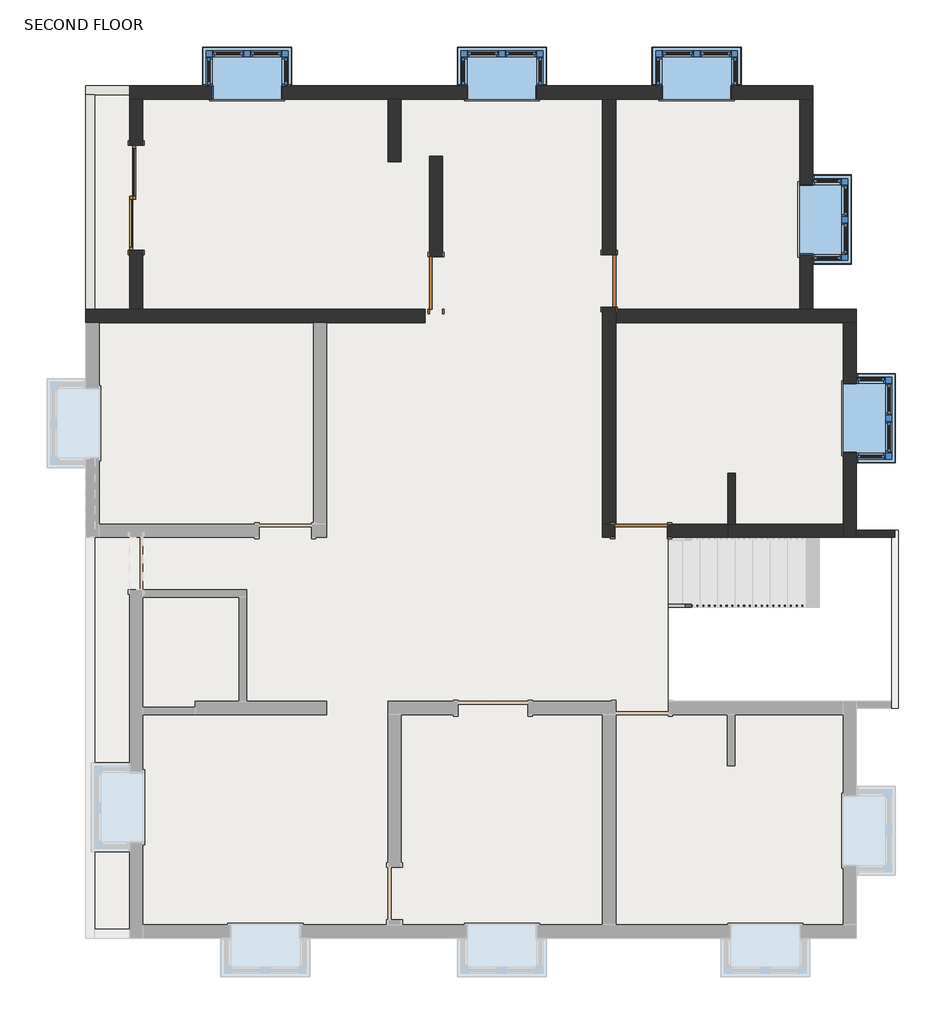
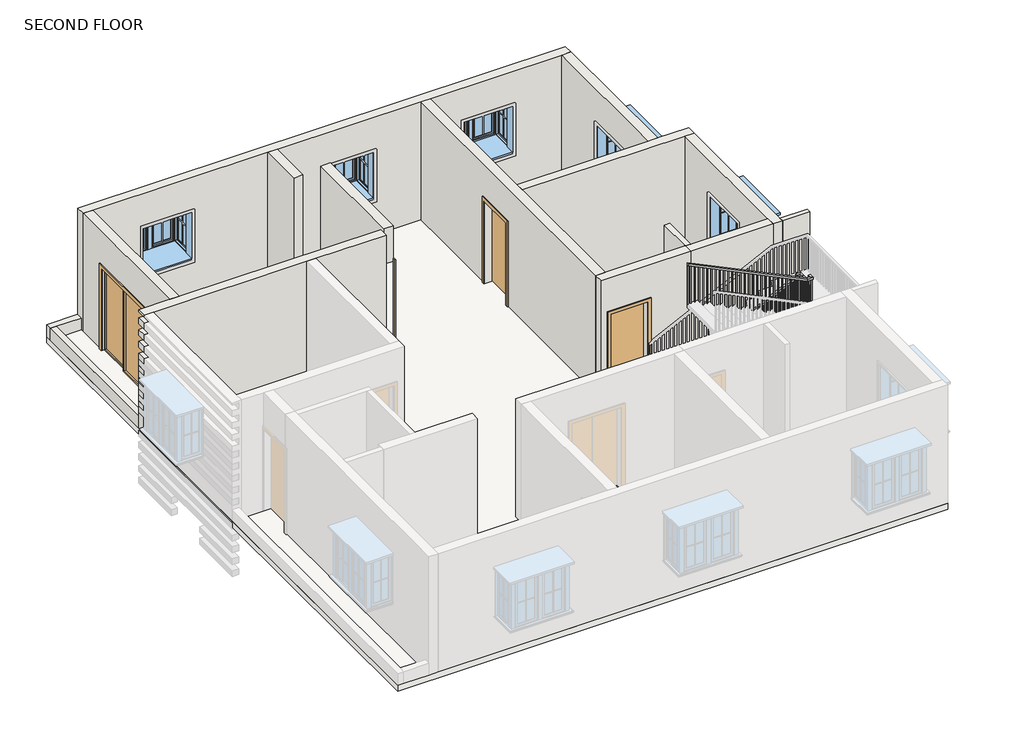
# One storey, part 2 of 6: 15 walls, 5 windows, 4 doors, 1 railing, 1 slab.
"""IFC4 building model written with IfcOpenShell, lengths in millimetres."""

from ifc_helpers import new_model, si_unit, frame, origin, place, context, project, spatial, polyline, outline, extrude, faceted_brep, transform, mapped, element, save
from components import door_d4d75d1e, door_a90ba1ad, door_0ca8825f, window_bay_casement_box_90_degree_angle_4_x4_x2_07b705a1

model = new_model("IFC4")

# Units and contexts
model_context = context("Model", 3, world=origin())
ifc_project = project(units=[si_unit("LENGTHUNIT", "METRE", prefix="MILLI")], contexts=[model_context])

# Site, building, storey
site = spatial("IfcSite", under=ifc_project)
building = spatial("IfcBuilding", under=site)
storey = spatial("IfcBuildingStorey", under=building, Name="SECOND FLOOR", Elevation=6400.8)

# Doors
placement = place(None, origin())
door_shape = door_d4d75d1e(model_context)
element("IfcDoor", 1, ObjectType="Door-Double-Sliding : 72\" x 84\"", at=placement, inside=storey, context=model_context, shape_type="MappedRepresentation", body=[
    mapped(door_shape, transform((-6005.0415084, 6126.233346, 6400.8), x_axis=(0.0, 1.0, 0.0), y_axis=(-1.0, 0.0, 0.0), z_axis=(0.0, 0.0, 1.0))),
])
door_2_shape = door_a90ba1ad(model_context)
element("IfcDoor", 2, ObjectType="Single-Flush : 36\" x 84\"", at=placement, inside=storey, context=model_context, shape_type="MappedRepresentation", body=[
    mapped(door_2_shape, transform((2656.3584916, 335.033346, 6400.8), x_axis=(-1.0, 0.0, 0.0), y_axis=(0.0, -1.0, 0.0), z_axis=(0.0, 0.0, 1.0))),
])
element("IfcDoor", 3, ObjectType="Single-Flush : 36\" x 84\"", at=placement, inside=storey, context=model_context, shape_type="MappedRepresentation", body=[
    mapped(door_2_shape, transform((-918.5024437, 4640.333346, 6400.8), x_axis=(0.0, -1.0, 0.0), y_axis=(1.0, 0.0, 0.0), z_axis=(0.0, 0.0, 1.0))),
])
door_3_shape = door_0ca8825f(model_context)
element("IfcDoor", 4, ObjectType="Single-Flush : 36\" x 84\"", at=placement, inside=storey, context=model_context, shape_type="MappedRepresentation", body=[
    mapped(door_3_shape, transform((2097.5584916, 4678.433346, 6400.8), x_axis=(0.0, -1.0, 0.0), y_axis=(1.0, 0.0, 0.0), z_axis=(0.0, 0.0, 1.0))),
])

# Railing
element("IfcRailing", 5, ObjectType="Handrail - Rectangular", at=placement, inside=storey, context=model_context, shape_type="SolidModel", body=[
    faceted_brep([(3126.2584916, -947.666654, 7460.6727273), (3126.2584916, -947.666654, 7404.1956113), (3126.2584916, -998.466654, 7404.1956113), (3126.2584916, -998.466654, 7460.6727273), (6044.5829507, -947.666654, 8878.3823634), (6095.3829507, -947.666654, 8846.5836718), (6095.3829507, -998.466654, 8846.5836718), (6044.5829507, -998.466654, 8878.3823634), (6044.5829507, -947.666654, 8915.4), (6095.3829507, -947.666654, 8864.6), (6095.3829507, -998.466654, 8864.6), (6044.5829507, -998.466654, 8915.4), (6171.5829507, -947.666654, 8915.4), (6171.5829507, -947.666654, 8864.6), (6120.7829507, -998.466654, 8864.6), (6120.7829507, -998.466654, 8915.4), (6171.5829507, -1074.666654, 8915.4), (6171.5829507, -1074.666654, 8864.6), (6120.7829507, -1074.666654, 8864.6), (6120.7829507, -1074.666654, 8915.4), (6171.5829507, -1341.366654, 8915.4), (6171.5829507, -1392.166654, 8864.6), (6120.7829507, -1392.166654, 8864.6), (6120.7829507, -1341.366654, 8915.4), (6171.5829507, -1341.366654, 9097.8903639), (6171.5829507, -1392.166654, 9047.0903639), (6120.7829507, -1392.166654, 9047.0903639), (6120.7829507, -1341.366654, 9097.8903639), (6171.5829507, -1468.366654, 9097.8903639), (6171.5829507, -1468.366654, 9047.0903639), (6120.7829507, -1417.566654, 9047.0903639), (6120.7829507, -1417.566654, 9097.8903639), (6044.5829507, -1468.366654, 9097.8903639), (6032.8967309, -1468.366654, 9047.0903639), (6032.8967309, -1417.566654, 9047.0903639), (6044.5829507, -1417.566654, 9097.8903639), (3126.2584916, -1468.366654, 10515.6), (3126.2584916, -1417.566654, 10515.6), (3126.2584916, -1417.566654, 10459.122884), (3126.2584916, -1468.366654, 10459.122884)], [[[0, 1, 2, 3]], [[1, 0, 4, 5]], [[2, 1, 5, 6]], [[3, 2, 6, 7]], [[0, 3, 7, 4]], [[5, 4, 8, 9]], [[6, 5, 9, 10]], [[7, 6, 10, 11]], [[4, 7, 11, 8]], [[9, 8, 12, 13]], [[10, 9, 13, 14]], [[11, 10, 14, 15]], [[8, 11, 15, 12]], [[13, 12, 16, 17]], [[14, 13, 17, 18]], [[15, 14, 18, 19]], [[12, 15, 19, 16]], [[17, 16, 20, 21]], [[18, 17, 21, 22]], [[19, 18, 22, 23]], [[16, 19, 23, 20]], [[21, 20, 24, 25]], [[22, 21, 25, 26]], [[23, 22, 26, 27]], [[20, 23, 27, 24]], [[25, 24, 28, 29]], [[26, 25, 29, 30]], [[27, 26, 30, 31]], [[24, 27, 31, 28]], [[29, 28, 32, 33]], [[30, 29, 33, 34]], [[31, 30, 34, 35]], [[28, 31, 35, 32]], [[36, 37, 38, 39]], [[33, 32, 36, 39]], [[34, 33, 39, 38]], [[35, 34, 38, 37]], [[32, 35, 37, 36]]]),
    extrude(outline(polyline([(10418.7778093, 3209.3079507), (10428.0322184, 3190.2579507), (9455.7272727, 3190.2579507), (9455.7272727, 3209.3079507), (10418.7778093, 3209.3079507)])), frame((0.0, -1452.491654, 0.0), z_axis=(0.0, 1.0, 0.0), x_axis=(0.0, 0.0, 1.0)), (0.0, 0.0, 1.0), 19.05),
    extrude(outline(polyline([(10369.4209605, 3310.9079507), (10378.6753696, 3291.8579507), (9455.7272727, 3291.8579507), (9455.7272727, 3310.9079507), (10369.4209605, 3310.9079507)])), frame((0.0, -1452.491654, 0.0), z_axis=(0.0, 1.0, 0.0), x_axis=(0.0, 0.0, 1.0)), (0.0, 0.0, 1.0), 19.05),
    extrude(outline(polyline([(10320.0641117, 3412.5079507), (10329.3185208, 3393.4579507), (9310.2545455, 3393.4579507), (9310.2545455, 3412.5079507), (10320.0641117, 3412.5079507)])), frame((0.0, -1452.491654, 0.0), z_axis=(0.0, 1.0, 0.0), x_axis=(0.0, 0.0, 1.0)), (0.0, 0.0, 1.0), 19.05),
    extrude(outline(polyline([(10270.7072629, 3514.1079507), (10279.9616721, 3495.0579507), (9310.2545455, 3495.0579507), (9310.2545455, 3514.1079507), (10270.7072629, 3514.1079507)])), frame((0.0, -1452.491654, 0.0), z_axis=(0.0, 1.0, 0.0), x_axis=(0.0, 0.0, 1.0)), (0.0, 0.0, 1.0), 19.05),
    extrude(outline(polyline([(10221.3504141, 3615.7079507), (10230.6048233, 3596.6579507), (9310.2545455, 3596.6579507), (9310.2545455, 3615.7079507), (10221.3504141, 3615.7079507)])), frame((0.0, -1452.491654, 0.0), z_axis=(0.0, 1.0, 0.0), x_axis=(0.0, 0.0, 1.0)), (0.0, 0.0, 1.0), 19.05),
    extrude(outline(polyline([(10171.9935653, 3717.3079507), (10181.2479745, 3698.2579507), (9164.7818182, 3698.2579507), (9164.7818182, 3717.3079507), (10171.9935653, 3717.3079507)])), frame((0.0, -1452.491654, 0.0), z_axis=(0.0, 1.0, 0.0), x_axis=(0.0, 0.0, 1.0)), (0.0, 0.0, 1.0), 19.05),
    extrude(outline(polyline([(10122.6367166, 3818.9079507), (10131.8911257, 3799.8579507), (9164.7818182, 3799.8579507), (9164.7818182, 3818.9079507), (10122.6367166, 3818.9079507)])), frame((0.0, -1452.491654, 0.0), z_axis=(0.0, 1.0, 0.0), x_axis=(0.0, 0.0, 1.0)), (0.0, 0.0, 1.0), 19.05),
    extrude(outline(polyline([(10073.2798678, 3920.5079507), (10082.5342769, 3901.4579507), (9164.7818182, 3901.4579507), (9164.7818182, 3920.5079507), (10073.2798678, 3920.5079507)])), frame((0.0, -1452.491654, 0.0), z_axis=(0.0, 1.0, 0.0), x_axis=(0.0, 0.0, 1.0)), (0.0, 0.0, 1.0), 19.05),
    extrude(outline(polyline([(10023.923019, 4022.1079507), (10033.1774281, 4003.0579507), (9019.3090909, 4003.0579507), (9019.3090909, 4022.1079507), (10023.923019, 4022.1079507)])), frame((0.0, -1452.491654, 0.0), z_axis=(0.0, 1.0, 0.0), x_axis=(0.0, 0.0, 1.0)), (0.0, 0.0, 1.0), 19.05),
    extrude(outline(polyline([(9974.5661702, 4123.7079507), (9983.8205793, 4104.6579507), (9019.3090909, 4104.6579507), (9019.3090909, 4123.7079507), (9974.5661702, 4123.7079507)])), frame((0.0, -1452.491654, 0.0), z_axis=(0.0, 1.0, 0.0), x_axis=(0.0, 0.0, 1.0)), (0.0, 0.0, 1.0), 19.05),
    extrude(outline(polyline([(9925.2093214, 4225.3079507), (9934.4637306, 4206.2579507), (9019.3090909, 4206.2579507), (9019.3090909, 4225.3079507), (9925.2093214, 4225.3079507)])), frame((0.0, -1452.491654, 0.0), z_axis=(0.0, 1.0, 0.0), x_axis=(0.0, 0.0, 1.0)), (0.0, 0.0, 1.0), 19.05),
    extrude(outline(polyline([(9875.8524726, 4326.9079507), (9885.1068818, 4307.8579507), (8873.8363636, 4307.8579507), (8873.8363636, 4326.9079507), (9875.8524726, 4326.9079507)])), frame((0.0, -1452.491654, 0.0), z_axis=(0.0, 1.0, 0.0), x_axis=(0.0, 0.0, 1.0)), (0.0, 0.0, 1.0), 19.05),
    extrude(outline(polyline([(9826.4956238, 4428.5079507), (9835.750033, 4409.4579507), (8873.8363636, 4409.4579507), (8873.8363636, 4428.5079507), (9826.4956238, 4428.5079507)])), frame((0.0, -1452.491654, 0.0), z_axis=(0.0, 1.0, 0.0), x_axis=(0.0, 0.0, 1.0)), (0.0, 0.0, 1.0), 19.05),
    extrude(outline(polyline([(9777.1387751, 4530.1079507), (9786.3931842, 4511.0579507), (8873.8363636, 4511.0579507), (8873.8363636, 4530.1079507), (9777.1387751, 4530.1079507)])), frame((0.0, -1452.491654, 0.0), z_axis=(0.0, 1.0, 0.0), x_axis=(0.0, 0.0, 1.0)), (0.0, 0.0, 1.0), 19.05),
    extrude(outline(polyline([(9727.7819263, 4631.7079507), (9737.0363354, 4612.6579507), (8728.3636364, 4612.6579507), (8728.3636364, 4631.7079507), (9727.7819263, 4631.7079507)])), frame((0.0, -1452.491654, 0.0), z_axis=(0.0, 1.0, 0.0), x_axis=(0.0, 0.0, 1.0)), (0.0, 0.0, 1.0), 19.05),
    extrude(outline(polyline([(9678.4250775, 4733.3079507), (9687.6794866, 4714.2579507), (8728.3636364, 4714.2579507), (8728.3636364, 4733.3079507), (9678.4250775, 4733.3079507)])), frame((0.0, -1452.491654, 0.0), z_axis=(0.0, 1.0, 0.0), x_axis=(0.0, 0.0, 1.0)), (0.0, 0.0, 1.0), 19.05),
    extrude(outline(polyline([(9629.0682287, 4834.9079507), (9638.3226379, 4815.8579507), (8728.3636364, 4815.8579507), (8728.3636364, 4834.9079507), (9629.0682287, 4834.9079507)])), frame((0.0, -1452.491654, 0.0), z_axis=(0.0, 1.0, 0.0), x_axis=(0.0, 0.0, 1.0)), (0.0, 0.0, 1.0), 19.05),
    extrude(outline(polyline([(9579.7113799, 4936.5079507), (9588.9657891, 4917.4579507), (8582.8909091, 4917.4579507), (8582.8909091, 4936.5079507), (9579.7113799, 4936.5079507)])), frame((0.0, -1452.491654, 0.0), z_axis=(0.0, 1.0, 0.0), x_axis=(0.0, 0.0, 1.0)), (0.0, 0.0, 1.0), 19.05),
    extrude(outline(polyline([(9530.3545311, 5038.1079507), (9539.6089403, 5019.0579507), (8582.8909091, 5019.0579507), (8582.8909091, 5038.1079507), (9530.3545311, 5038.1079507)])), frame((0.0, -1452.491654, 0.0), z_axis=(0.0, 1.0, 0.0), x_axis=(0.0, 0.0, 1.0)), (0.0, 0.0, 1.0), 19.05),
    extrude(outline(polyline([(9480.9976824, 5139.7079507), (9490.2520915, 5120.6579507), (8582.8909091, 5120.6579507), (8582.8909091, 5139.7079507), (9480.9976824, 5139.7079507)])), frame((0.0, -1452.491654, 0.0), z_axis=(0.0, 1.0, 0.0), x_axis=(0.0, 0.0, 1.0)), (0.0, 0.0, 1.0), 19.05),
    extrude(outline(polyline([(9431.559384, 5241.3079507), (9440.8137931, 5222.2579507), (8437.4181818, 5222.2579507), (8437.4181818, 5241.3079507), (9431.559384, 5241.3079507)])), frame((0.0, -1452.491654, 0.0), z_axis=(0.0, 1.0, 0.0), x_axis=(0.0, 0.0, 1.0)), (0.0, 0.0, 1.0), 19.05),
    extrude(outline(polyline([(9382.2839848, 5342.9079507), (9391.5383939, 5323.8579507), (8437.4181818, 5323.8579507), (8437.4181818, 5342.9079507), (9382.2839848, 5342.9079507)])), frame((0.0, -1452.491654, 0.0), z_axis=(0.0, 1.0, 0.0), x_axis=(0.0, 0.0, 1.0)), (0.0, 0.0, 1.0), 19.05),
    extrude(outline(polyline([(9332.927136, 5444.5079507), (9342.1815452, 5425.4579507), (8437.4181818, 5425.4579507), (8437.4181818, 5444.5079507), (9332.927136, 5444.5079507)])), frame((0.0, -1452.491654, 0.0), z_axis=(0.0, 1.0, 0.0), x_axis=(0.0, 0.0, 1.0)), (0.0, 0.0, 1.0), 19.05),
    extrude(outline(polyline([(9283.5702872, 5546.1079507), (9292.8246964, 5527.0579507), (8291.9454545, 5527.0579507), (8291.9454545, 5546.1079507), (9283.5702872, 5546.1079507)])), frame((0.0, -1452.491654, 0.0), z_axis=(0.0, 1.0, 0.0), x_axis=(0.0, 0.0, 1.0)), (0.0, 0.0, 1.0), 19.05),
    extrude(outline(polyline([(9234.2134384, 5647.7079507), (9243.4678476, 5628.6579507), (8291.9454545, 5628.6579507), (8291.9454545, 5647.7079507), (9234.2134384, 5647.7079507)])), frame((0.0, -1452.491654, 0.0), z_axis=(0.0, 1.0, 0.0), x_axis=(0.0, 0.0, 1.0)), (0.0, 0.0, 1.0), 19.05),
    extrude(outline(polyline([(9184.8565897, 5749.3079507), (9194.1109988, 5730.2579507), (8291.9454545, 5730.2579507), (8291.9454545, 5749.3079507), (9184.8565897, 5749.3079507)])), frame((0.0, -1452.491654, 0.0), z_axis=(0.0, 1.0, 0.0), x_axis=(0.0, 0.0, 1.0)), (0.0, 0.0, 1.0), 19.05),
    extrude(outline(polyline([(9135.4997409, 5850.9079507), (9144.75415, 5831.8579507), (8146.4727273, 5831.8579507), (8146.4727273, 5850.9079507), (9135.4997409, 5850.9079507)])), frame((0.0, -1452.491654, 0.0), z_axis=(0.0, 1.0, 0.0), x_axis=(0.0, 0.0, 1.0)), (0.0, 0.0, 1.0), 19.05),
    extrude(outline(polyline([(9086.1428921, 5952.5079507), (9095.3973012, 5933.4579507), (8146.4727273, 5933.4579507), (8146.4727273, 5952.5079507), (9086.1428921, 5952.5079507)])), frame((0.0, -1452.491654, 0.0), z_axis=(0.0, 1.0, 0.0), x_axis=(0.0, 0.0, 1.0)), (0.0, 0.0, 1.0), 19.05),
    extrude(outline(polyline([(9036.7860433, 6054.1079507), (9046.0404524, 6035.0579507), (8146.4727273, 6035.0579507), (8146.4727273, 6054.1079507), (9036.7860433, 6054.1079507)])), frame((0.0, -1452.491654, 0.0), z_axis=(0.0, 1.0, 0.0), x_axis=(0.0, 0.0, 1.0)), (0.0, 0.0, 1.0), 19.05),
    extrude(outline(polyline([(6136.6579507, -1369.941654), (6155.7079507, -1369.941654), (6155.7079507, -1388.991654), (6136.6579507, -1388.991654), (6136.6579507, -1369.941654)])), frame((0.0, 0.0, 8001.0), z_axis=(0.0, 0.0, 1.0), x_axis=(1.0, 0.0, 0.0)), (0.0, 0.0, 1.0), 1046.0903639),
    extrude(outline(polyline([(6136.6579507, -1268.341654), (6155.7079507, -1268.341654), (6155.7079507, -1287.391654), (6136.6579507, -1287.391654), (6136.6579507, -1268.341654)])), frame((0.0, 0.0, 8001.0), z_axis=(0.0, 0.0, 1.0), x_axis=(1.0, 0.0, 0.0)), (0.0, 0.0, 1.0), 863.6),
    extrude(outline(polyline([(6136.6579507, -1166.741654), (6155.7079507, -1166.741654), (6155.7079507, -1185.791654), (6136.6579507, -1185.791654), (6136.6579507, -1166.741654)])), frame((0.0, 0.0, 8001.0), z_axis=(0.0, 0.0, 1.0), x_axis=(1.0, 0.0, 0.0)), (0.0, 0.0, 1.0), 863.6),
    extrude(outline(polyline([(6136.6579507, -1065.141654), (6155.7079507, -1065.141654), (6155.7079507, -1084.191654), (6136.6579507, -1084.191654), (6136.6579507, -1065.141654)])), frame((0.0, 0.0, 8001.0), z_axis=(0.0, 0.0, 1.0), x_axis=(1.0, 0.0, 0.0)), (0.0, 0.0, 1.0), 863.6),
    extrude(outline(polyline([(6063.1334916, -982.591654), (6063.1334916, -963.541654), (6082.1834916, -963.541654), (6082.1834916, -982.591654), (6063.1334916, -982.591654)])), frame((0.0, 0.0, 7855.5272727), z_axis=(0.0, 0.0, 1.0), x_axis=(1.0, 0.0, 0.0)), (0.0, 0.0, 1.0), 1009.0727273),
    extrude(outline(polyline([(8790.8145818, 5980.5834916), (8781.5601727, 5961.5334916), (7855.5272727, 5961.5334916), (7855.5272727, 5980.5834916), (8790.8145818, 5980.5834916)])), frame((0.0, -982.591654, 0.0), z_axis=(0.0, 1.0, 0.0), x_axis=(0.0, 0.0, 1.0)), (0.0, 0.0, 1.0), 19.05),
    extrude(outline(polyline([(8741.457733, 5878.9834916), (8732.2033239, 5859.9334916), (7855.5272727, 5859.9334916), (7855.5272727, 5878.9834916), (8741.457733, 5878.9834916)])), frame((0.0, -982.591654, 0.0), z_axis=(0.0, 1.0, 0.0), x_axis=(0.0, 0.0, 1.0)), (0.0, 0.0, 1.0), 19.05),
    extrude(outline(polyline([(8692.1008843, 5777.3834916), (8682.8464751, 5758.3334916), (7710.0545455, 5758.3334916), (7710.0545455, 5777.3834916), (8692.1008843, 5777.3834916)])), frame((0.0, -982.591654, 0.0), z_axis=(0.0, 1.0, 0.0), x_axis=(0.0, 0.0, 1.0)), (0.0, 0.0, 1.0), 19.05),
    extrude(outline(polyline([(8642.7440355, 5675.7834916), (8633.4896263, 5656.7334916), (7710.0545455, 5656.7334916), (7710.0545455, 5675.7834916), (8642.7440355, 5675.7834916)])), frame((0.0, -982.591654, 0.0), z_axis=(0.0, 1.0, 0.0), x_axis=(0.0, 0.0, 1.0)), (0.0, 0.0, 1.0), 19.05),
    extrude(outline(polyline([(8593.3871867, 5574.1834916), (8584.1327775, 5555.1334916), (7710.0545455, 5555.1334916), (7710.0545455, 5574.1834916), (8593.3871867, 5574.1834916)])), frame((0.0, -982.591654, 0.0), z_axis=(0.0, 1.0, 0.0), x_axis=(0.0, 0.0, 1.0)), (0.0, 0.0, 1.0), 19.05),
    extrude(outline(polyline([(8544.0303379, 5472.5834916), (8534.7759288, 5453.5334916), (7564.5818182, 5453.5334916), (7564.5818182, 5472.5834916), (8544.0303379, 5472.5834916)])), frame((0.0, -982.591654, 0.0), z_axis=(0.0, 1.0, 0.0), x_axis=(0.0, 0.0, 1.0)), (0.0, 0.0, 1.0), 19.05),
    extrude(outline(polyline([(8494.6734891, 5370.9834916), (8485.41908, 5351.9334916), (7564.5818182, 5351.9334916), (7564.5818182, 5370.9834916), (8494.6734891, 5370.9834916)])), frame((0.0, -982.591654, 0.0), z_axis=(0.0, 1.0, 0.0), x_axis=(0.0, 0.0, 1.0)), (0.0, 0.0, 1.0), 19.05),
    extrude(outline(polyline([(8445.3166403, 5269.3834916), (8436.0622312, 5250.3334916), (7564.5818182, 5250.3334916), (7564.5818182, 5269.3834916), (8445.3166403, 5269.3834916)])), frame((0.0, -982.591654, 0.0), z_axis=(0.0, 1.0, 0.0), x_axis=(0.0, 0.0, 1.0)), (0.0, 0.0, 1.0), 19.05),
    extrude(outline(polyline([(8395.9597915, 5167.7834916), (8386.7053824, 5148.7334916), (7419.1090909, 5148.7334916), (7419.1090909, 5167.7834916), (8395.9597915, 5167.7834916)])), frame((0.0, -982.591654, 0.0), z_axis=(0.0, 1.0, 0.0), x_axis=(0.0, 0.0, 1.0)), (0.0, 0.0, 1.0), 19.05),
    extrude(outline(polyline([(8346.6029428, 5066.1834916), (8337.3485336, 5047.1334916), (7419.1090909, 5047.1334916), (7419.1090909, 5066.1834916), (8346.6029428, 5066.1834916)])), frame((0.0, -982.591654, 0.0), z_axis=(0.0, 1.0, 0.0), x_axis=(0.0, 0.0, 1.0)), (0.0, 0.0, 1.0), 19.05),
    extrude(outline(polyline([(8297.246094, 4964.5834916), (8287.9916848, 4945.5334916), (7419.1090909, 4945.5334916), (7419.1090909, 4964.5834916), (8297.246094, 4964.5834916)])), frame((0.0, -982.591654, 0.0), z_axis=(0.0, 1.0, 0.0), x_axis=(0.0, 0.0, 1.0)), (0.0, 0.0, 1.0), 19.05),
    extrude(outline(polyline([(8247.8892452, 4862.9834916), (8238.634836, 4843.9334916), (7273.6363636, 4843.9334916), (7273.6363636, 4862.9834916), (8247.8892452, 4862.9834916)])), frame((0.0, -982.591654, 0.0), z_axis=(0.0, 1.0, 0.0), x_axis=(0.0, 0.0, 1.0)), (0.0, 0.0, 1.0), 19.05),
    extrude(outline(polyline([(8198.5323964, 4761.3834916), (8189.2779873, 4742.3334916), (7273.6363636, 4742.3334916), (7273.6363636, 4761.3834916), (8198.5323964, 4761.3834916)])), frame((0.0, -982.591654, 0.0), z_axis=(0.0, 1.0, 0.0), x_axis=(0.0, 0.0, 1.0)), (0.0, 0.0, 1.0), 19.05),
    extrude(outline(polyline([(8149.1755476, 4659.7834916), (8139.9211385, 4640.7334916), (7273.6363636, 4640.7334916), (7273.6363636, 4659.7834916), (8149.1755476, 4659.7834916)])), frame((0.0, -982.591654, 0.0), z_axis=(0.0, 1.0, 0.0), x_axis=(0.0, 0.0, 1.0)), (0.0, 0.0, 1.0), 19.05),
    extrude(outline(polyline([(8099.8186988, 4558.1834916), (8090.5642897, 4539.1334916), (7128.1636364, 4539.1334916), (7128.1636364, 4558.1834916), (8099.8186988, 4558.1834916)])), frame((0.0, -982.591654, 0.0), z_axis=(0.0, 1.0, 0.0), x_axis=(0.0, 0.0, 1.0)), (0.0, 0.0, 1.0), 19.05),
    extrude(outline(polyline([(8050.4618501, 4456.5834916), (8041.2074409, 4437.5334916), (7128.1636364, 4437.5334916), (7128.1636364, 4456.5834916), (8050.4618501, 4456.5834916)])), frame((0.0, -982.591654, 0.0), z_axis=(0.0, 1.0, 0.0), x_axis=(0.0, 0.0, 1.0)), (0.0, 0.0, 1.0), 19.05),
    extrude(outline(polyline([(8001.1050013, 4354.9834916), (7991.8505921, 4335.9334916), (7128.1636364, 4335.9334916), (7128.1636364, 4354.9834916), (8001.1050013, 4354.9834916)])), frame((0.0, -982.591654, 0.0), z_axis=(0.0, 1.0, 0.0), x_axis=(0.0, 0.0, 1.0)), (0.0, 0.0, 1.0), 19.05),
    extrude(outline(polyline([(7951.7481525, 4253.3834916), (7942.4937433, 4234.3334916), (6982.6909091, 4234.3334916), (6982.6909091, 4253.3834916), (7951.7481525, 4253.3834916)])), frame((0.0, -982.591654, 0.0), z_axis=(0.0, 1.0, 0.0), x_axis=(0.0, 0.0, 1.0)), (0.0, 0.0, 1.0), 19.05),
    extrude(outline(polyline([(7902.3913037, 4151.7834916), (7893.1368946, 4132.7334916), (6982.6909091, 4132.7334916), (6982.6909091, 4151.7834916), (7902.3913037, 4151.7834916)])), frame((0.0, -982.591654, 0.0), z_axis=(0.0, 1.0, 0.0), x_axis=(0.0, 0.0, 1.0)), (0.0, 0.0, 1.0), 19.05),
    extrude(outline(polyline([(7853.0344549, 4050.1834916), (7843.7800458, 4031.1334916), (6982.6909091, 4031.1334916), (6982.6909091, 4050.1834916), (7853.0344549, 4050.1834916)])), frame((0.0, -982.591654, 0.0), z_axis=(0.0, 1.0, 0.0), x_axis=(0.0, 0.0, 1.0)), (0.0, 0.0, 1.0), 19.05),
    extrude(outline(polyline([(7803.6776061, 3948.5834916), (7794.423197, 3929.5334916), (6837.2181818, 3929.5334916), (6837.2181818, 3948.5834916), (7803.6776061, 3948.5834916)])), frame((0.0, -982.591654, 0.0), z_axis=(0.0, 1.0, 0.0), x_axis=(0.0, 0.0, 1.0)), (0.0, 0.0, 1.0), 19.05),
    extrude(outline(polyline([(7754.3207573, 3846.9834916), (7745.0663482, 3827.9334916), (6837.2181818, 3827.9334916), (6837.2181818, 3846.9834916), (7754.3207573, 3846.9834916)])), frame((0.0, -982.591654, 0.0), z_axis=(0.0, 1.0, 0.0), x_axis=(0.0, 0.0, 1.0)), (0.0, 0.0, 1.0), 19.05),
    extrude(outline(polyline([(7704.9639086, 3745.3834916), (7695.7094994, 3726.3334916), (6837.2181818, 3726.3334916), (6837.2181818, 3745.3834916), (7704.9639086, 3745.3834916)])), frame((0.0, -982.591654, 0.0), z_axis=(0.0, 1.0, 0.0), x_axis=(0.0, 0.0, 1.0)), (0.0, 0.0, 1.0), 19.05),
    extrude(outline(polyline([(7655.6070598, 3643.7834916), (7646.3526506, 3624.7334916), (6691.7454545, 3624.7334916), (6691.7454545, 3643.7834916), (7655.6070598, 3643.7834916)])), frame((0.0, -982.591654, 0.0), z_axis=(0.0, 1.0, 0.0), x_axis=(0.0, 0.0, 1.0)), (0.0, 0.0, 1.0), 19.05),
    extrude(outline(polyline([(7606.250211, 3542.1834916), (7596.9958018, 3523.1334916), (6691.7454545, 3523.1334916), (6691.7454545, 3542.1834916), (7606.250211, 3542.1834916)])), frame((0.0, -982.591654, 0.0), z_axis=(0.0, 1.0, 0.0), x_axis=(0.0, 0.0, 1.0)), (0.0, 0.0, 1.0), 19.05),
    extrude(outline(polyline([(7556.8933622, 3440.5834916), (7547.6389531, 3421.5334916), (6691.7454545, 3421.5334916), (6691.7454545, 3440.5834916), (7556.8933622, 3440.5834916)])), frame((0.0, -982.591654, 0.0), z_axis=(0.0, 1.0, 0.0), x_axis=(0.0, 0.0, 1.0)), (0.0, 0.0, 1.0), 19.05),
    extrude(outline(polyline([(7507.5365134, 3338.9834916), (7498.2821043, 3319.9334916), (6546.2727273, 3319.9334916), (6546.2727273, 3338.9834916), (7507.5365134, 3338.9834916)])), frame((0.0, -982.591654, 0.0), z_axis=(0.0, 1.0, 0.0), x_axis=(0.0, 0.0, 1.0)), (0.0, 0.0, 1.0), 19.05),
    extrude(outline(polyline([(7458.1796646, 3237.3834916), (7448.9252555, 3218.3334916), (6546.2727273, 3218.3334916), (6546.2727273, 3237.3834916), (7458.1796646, 3237.3834916)])), frame((0.0, -982.591654, 0.0), z_axis=(0.0, 1.0, 0.0), x_axis=(0.0, 0.0, 1.0)), (0.0, 0.0, 1.0), 19.05),
    extrude(outline(polyline([(6136.6579507, -1433.441654), (6155.7079507, -1433.441654), (6155.7079507, -1452.491654), (6136.6579507, -1452.491654), (6136.6579507, -1433.441654)])), frame((0.0, 0.0, 8001.0), z_axis=(0.0, 0.0, 1.0), x_axis=(1.0, 0.0, 0.0)), (0.0, 0.0, 1.0), 1046.0903639),
    extrude(outline(polyline([(6136.6579507, -982.591654), (6136.6579507, -963.541654), (6155.7079507, -963.541654), (6155.7079507, -982.591654), (6136.6579507, -982.591654)])), frame((0.0, 0.0, 8001.0), z_axis=(0.0, 0.0, 1.0), x_axis=(1.0, 0.0, 0.0)), (0.0, 0.0, 1.0), 863.6),
    extrude(outline(polyline([(10449.8684749, 3145.3084916), (10459.122884, 3126.2584916), (9455.7272727, 3126.2584916), (9455.7272727, 3145.3084916), (10449.8684749, 3145.3084916)])), frame((0.0, -1452.491654, 0.0), z_axis=(0.0, 1.0, 0.0), x_axis=(0.0, 0.0, 1.0)), (0.0, 0.0, 1.0), 19.05),
    extrude(outline(polyline([(7413.4500204, 3145.3084916), (7404.1956113, 3126.2584916), (6546.2727273, 3126.2584916), (6546.2727273, 3145.3084916), (7413.4500204, 3145.3084916)])), frame((0.0, -982.591654, 0.0), z_axis=(0.0, 1.0, 0.0), x_axis=(0.0, 0.0, 1.0)), (0.0, 0.0, 1.0), 19.05),
])

# Slab
element("IfcSlab", 6, ObjectType="6\"", at=placement, inside=storey, context=model_context, shape_type="SweptSolid", body=[
    extrude(outline(polyline([(-7008.3415084, -6751.566654), (-7008.3415084, 220.733346), (-7008.3415084, 8069.333346), (5640.8584916, 8069.333346), (5640.8584916, 4183.133346), (6402.8584916, 4183.133346), (6402.8584916, 337.573346), (7125.9750459, 337.573346), (7125.9750459, -2753.606654), (6402.8584916, -2753.606654), (6402.8584916, -6751.566654), (-7008.3415084, -6751.566654)]), holes=[polyline([(7009.1350459, 220.733346), (3126.2584916, 220.733346), (3126.2584916, -2636.766654), (7009.1350459, -2636.766654), (7009.1350459, 220.733346)])]), frame((0.0, 0.0, 6248.4), z_axis=(0.0, 0.0, 1.0), x_axis=(1.0, 0.0, 0.0)), (0.0, 0.0, 1.0), 152.4),
])

# Walls
element("IfcWall", 7, ObjectType="4.6\"", at=placement, inside=storey, context=model_context, shape_type="SweptSolid", body=[
    extrude(outline(polyline([(7067.5550459, 220.733346), (6402.8584916, 220.733346), (6402.8584916, 337.573346), (7067.5550459, 337.573346), (7067.5550459, 220.733346)])), frame((0.0, 0.0, 6400.8), z_axis=(0.0, 0.0, 1.0), x_axis=(1.0, 0.0, 0.0)), (0.0, 0.0, 1.0), 3048.0),
])
element("IfcWall", 8, ObjectType="5\"", at=placement, inside=storey, context=model_context, shape_type="SweptSolid", body=[
    extrude(outline(polyline([(4291.9829507, 1335.1417393), (4291.9829507, 449.333346), (4164.9829507, 449.333346), (4164.9829507, 1335.1417393), (4291.9829507, 1335.1417393)])), frame((0.0, 0.0, 6400.8), z_axis=(0.0, 0.0, 1.0), x_axis=(1.0, 0.0, 0.0)), (0.0, 0.0, 1.0), 3048.0),
])
element("IfcWall", 9, ObjectType="6\"", at=placement, inside=storey, context=model_context, shape_type="Brep", body=[
    faceted_brep([(-6246.3415084, 8069.333346, 6400.8), (-7008.3415084, 8069.333346, 6400.8), (-7008.3415084, 8069.333346, 6705.6), (-6246.3415084, 8069.333346, 6705.6), (-6246.3415084, 7916.933346, 6400.8), (-6246.3415084, 7916.933346, 6705.6), (-6855.9415084, 7916.933346, 6705.6), (-7008.3415084, 7916.933346, 6705.6), (-7008.3415084, 7916.933346, 6400.8), (-6855.9415084, 7916.933346, 6400.8)], [[[0, 1, 2, 3]], [[4, 5, 6, 7, 8, 9]], [[1, 0, 4, 9, 8]], [[3, 2, 7, 6, 5]], [[2, 1, 8, 7]], [[0, 3, 5, 4]]]),
])
element("IfcWall", 10, ObjectType="6\"", at=placement, inside=storey, context=model_context, shape_type="SweptSolid", body=[
    extrude(outline(polyline([(-7008.3415084, 4183.133346), (-7008.3415084, 7916.933346), (-6855.9415084, 7916.933346), (-6855.9415084, 4183.133346), (-7008.3415084, 4183.133346)])), frame((0.0, 0.0, 6400.8), z_axis=(0.0, 0.0, 1.0), x_axis=(1.0, 0.0, 0.0)), (0.0, 0.0, 1.0), 304.8),
])
element("IfcWall", 11, ObjectType="9\"", at=placement, inside=storey, context=model_context, shape_type="Brep", body=[
    faceted_brep([(5640.8584916, 8069.333346, 6400.8), (-6246.3415084, 8069.333346, 6400.8), (-6246.3415084, 8069.333346, 6705.6), (-6246.3415084, 8069.333346, 9448.8), (5640.8584916, 8069.333346, 9448.8), (-3592.0415084, 8069.333346, 8585.2), (-4811.2415084, 8069.333346, 8585.2), (-4811.2415084, 8069.333346, 7315.2), (-3592.0415084, 8069.333346, 7315.2), (4231.1584916, 8069.333346, 8585.2), (3011.9584916, 8069.333346, 8585.2), (3011.9584916, 8069.333346, 7315.2), (4231.1584916, 8069.333346, 7315.2), (840.2584916, 8069.333346, 8585.2), (-378.9415084, 8069.333346, 8585.2), (-378.9415084, 8069.333346, 7315.2), (840.2584916, 8069.333346, 7315.2), (5640.8584916, 7840.733346, 6400.8), (5640.8584916, 7840.733346, 9448.8), (5412.2584916, 7840.733346, 9448.8), (2211.8584916, 7840.733346, 9448.8), (1983.2584916, 7840.733346, 9448.8), (-1521.9415084, 7840.733346, 9448.8), (-1750.5415084, 7840.733346, 9448.8), (-6017.7415084, 7840.733346, 9448.8), (-6246.3415084, 7840.733346, 9448.8), (-6246.3415084, 7840.733346, 6400.8), (-6017.7415084, 7840.733346, 6400.8), (-1750.5415084, 7840.733346, 6400.8), (-1521.9415084, 7840.733346, 6400.8), (1983.2584916, 7840.733346, 6400.8), (2211.8584916, 7840.733346, 6400.8), (5412.2584916, 7840.733346, 6400.8), (-3592.0415084, 7840.733346, 8585.2), (-3592.0415084, 7840.733346, 7315.2), (-4811.2415084, 7840.733346, 7315.2), (-4811.2415084, 7840.733346, 8585.2), (4231.1584916, 7840.733346, 8585.2), (4231.1584916, 7840.733346, 7315.2), (3011.9584916, 7840.733346, 7315.2), (3011.9584916, 7840.733346, 8585.2), (840.2584916, 7840.733346, 8585.2), (840.2584916, 7840.733346, 7315.2), (-378.9415084, 7840.733346, 7315.2), (-378.9415084, 7840.733346, 8585.2), (-6246.3415084, 7916.933346, 6400.8)], [[[0, 1, 2, 3, 4], [5, 6, 7, 8], [9, 10, 11, 12], [13, 14, 15, 16]], [[17, 18, 19, 20, 21, 22, 23, 24, 25, 26, 27, 28, 29, 30, 31, 32], [33, 34, 35, 36], [37, 38, 39, 40], [41, 42, 43, 44]], [[1, 0, 17, 32, 31, 30, 29, 28, 27, 26, 45]], [[4, 3, 25, 24, 23, 22, 21, 20, 19, 18]], [[0, 4, 18, 17]], [[34, 33, 5, 8]], [[35, 34, 8, 7]], [[36, 35, 7, 6]], [[33, 36, 6, 5]], [[38, 37, 9, 12]], [[39, 38, 12, 11]], [[40, 39, 11, 10]], [[37, 40, 10, 9]], [[42, 41, 13, 16]], [[43, 42, 16, 15]], [[44, 43, 15, 14]], [[41, 44, 14, 13]], [[1, 45, 26, 25, 3, 2]]]),
])
element("IfcWall", 12, ObjectType="9\"", at=placement, inside=storey, context=model_context, shape_type="SweptSolid", body=[
    extrude(outline(polyline([(7840.733346, 6400.8), (7040.633346, 6400.8), (7040.633346, 8534.4), (5211.833346, 8534.4), (5211.833346, 6400.8), (4183.133346, 6400.8), (4183.133346, 9448.8), (7840.733346, 9448.8), (7840.733346, 6400.8)])), frame((-6246.3415084, 0.0, 0.0), z_axis=(1.0, 0.0, 0.0), x_axis=(0.0, 1.0, 0.0)), (0.0, 0.0, 1.0), 228.6),
])
element("IfcWall", 13, ObjectType="9\"", at=placement, inside=storey, context=model_context, shape_type="SweptSolid", body=[
    extrude(outline(polyline([(7840.733346, 6400.8), (4183.133346, 6400.8), (4183.133346, 9448.8), (7840.733346, 9448.8), (7840.733346, 6400.8)]), holes=[polyline([(5135.633346, 8585.2), (5135.633346, 7315.2), (6354.833346, 7315.2), (6354.833346, 8585.2), (5135.633346, 8585.2)])]), frame((5412.2584916, 0.0, 0.0), z_axis=(1.0, 0.0, 0.0), x_axis=(0.0, 1.0, 0.0)), (0.0, 0.0, 1.0), 228.6),
])
element("IfcWall", 14, ObjectType="9\"", at=placement, inside=storey, context=model_context, shape_type="Brep", body=[
    faceted_brep([(1983.2584916, 4221.233346, 8534.4), (1983.2584916, 4221.233346, 6400.8), (1983.2584916, 449.333346, 6400.8), (1983.2584916, 449.333346, 9448.8), (1983.2584916, 7840.733346, 9448.8), (1983.2584916, 7840.733346, 6400.8), (1983.2584916, 5135.633346, 6400.8), (1983.2584916, 5135.633346, 8534.4), (2211.8584916, 449.333346, 6400.8), (2211.8584916, 3954.533346, 6400.8), (2211.8584916, 4183.133346, 6400.8), (2211.8584916, 4221.233346, 6400.8), (2211.8584916, 4221.233346, 8534.4), (2211.8584916, 5135.633346, 8534.4), (2211.8584916, 5135.633346, 6400.8), (2211.8584916, 7840.733346, 6400.8), (2211.8584916, 7840.733346, 9448.8), (2211.8584916, 4183.133346, 9448.8), (2211.8584916, 3954.533346, 9448.8), (2211.8584916, 449.333346, 9448.8), (2199.1584916, 449.333346, 6400.8)], [[[0, 1, 2, 3, 4, 5, 6, 7]], [[8, 9, 10, 11, 12, 13, 14, 15, 16, 17, 18, 19]], [[6, 5, 15, 14]], [[2, 1, 11, 10, 9, 8, 20]], [[4, 3, 19, 18, 17, 16]], [[5, 4, 16, 15]], [[3, 2, 20, 8, 19]], [[12, 11, 1, 0]], [[13, 12, 0, 7]], [[14, 13, 7, 6]]]),
])
element("IfcWall", 15, ObjectType="9\"", at=placement, inside=storey, context=model_context, shape_type="SweptSolid", body=[
    extrude(outline(polyline([(-1750.5415084, 6747.0175593), (-1750.5415084, 7840.733346), (-1521.9415084, 7840.733346), (-1521.9415084, 6747.0175593), (-1750.5415084, 6747.0175593)])), frame((0.0, 0.0, 6400.8), z_axis=(0.0, 0.0, 1.0), x_axis=(1.0, 0.0, 0.0)), (0.0, 0.0, 1.0), 3048.0),
])
element("IfcWall", 16, ObjectType="9\"", at=placement, inside=storey, context=model_context, shape_type="Brep", body=[
    faceted_brep([(-1108.4404612, 4183.133346, 6400.8), (-6017.7415084, 4183.133346, 6400.8), (-6246.3415084, 4183.133346, 6400.8), (-6855.9415084, 4183.133346, 6400.8), (-7008.3415084, 4183.133346, 6400.8), (-7008.3415084, 4183.133346, 6705.6), (-7008.3415084, 4183.133346, 6807.2), (-6855.9415084, 4183.133346, 6807.2), (-6855.9415084, 4183.133346, 6959.6), (-7008.3415084, 4183.133346, 6959.6), (-7008.3415084, 4183.133346, 7112.0), (-6855.9415084, 4183.133346, 7112.0), (-6855.9415084, 4183.133346, 7264.4), (-7008.3415084, 4183.133346, 7264.4), (-7008.3415084, 4183.133346, 7416.8), (-6855.9415084, 4183.133346, 7416.8), (-6855.9415084, 4183.133346, 7569.2), (-7008.3415084, 4183.133346, 7569.2), (-7008.3415084, 4183.133346, 7721.6), (-6855.9415084, 4183.133346, 7721.6), (-6855.9415084, 4183.133346, 7874.0), (-7008.3415084, 4183.133346, 7874.0), (-7008.3415084, 4183.133346, 8026.4), (-6855.9415084, 4183.133346, 8026.4), (-6855.9415084, 4183.133346, 8178.8), (-7008.3415084, 4183.133346, 8178.8), (-7008.3415084, 4183.133346, 8331.2), (-6855.9415084, 4183.133346, 8331.2), (-6855.9415084, 4183.133346, 8483.6), (-7008.3415084, 4183.133346, 8483.6), (-7008.3415084, 4183.133346, 8636.0), (-6855.9415084, 4183.133346, 8636.0), (-6855.9415084, 4183.133346, 8788.4), (-7008.3415084, 4183.133346, 8788.4), (-7008.3415084, 4183.133346, 8940.8), (-6855.9415084, 4183.133346, 8940.8), (-6855.9415084, 4183.133346, 9093.2), (-7008.3415084, 4183.133346, 9093.2), (-7008.3415084, 4183.133346, 9245.6), (-6855.9415084, 4183.133346, 9245.6), (-6855.9415084, 4183.133346, 9398.0), (-7008.3415084, 4183.133346, 9398.0), (-7008.3415084, 4183.133346, 9448.8), (-6246.3415084, 4183.133346, 9448.8), (-6017.7415084, 4183.133346, 9448.8), (-1108.4404612, 4183.133346, 9448.8), (-7008.3415084, 3954.533346, 6400.8), (-6779.7415084, 3954.533346, 6400.8), (-3045.9415084, 3954.533346, 6400.8), (-2817.3415084, 3954.533346, 6400.8), (-1108.4404612, 3954.533346, 6400.8), (-1108.4404612, 3954.533346, 9448.8), (-2817.3415084, 3954.533346, 9448.8), (-3045.9415084, 3954.533346, 9448.8), (-6779.7415084, 3954.533346, 9448.8), (-7008.3415084, 3954.533346, 9448.8), (-7008.3415084, 3954.533346, 9398.0), (-6855.9415084, 3954.533346, 9398.0), (-6855.9415084, 3954.533346, 9245.6), (-7008.3415084, 3954.533346, 9245.6), (-7008.3415084, 3954.533346, 9093.2), (-6855.9415084, 3954.533346, 9093.2), (-6855.9415084, 3954.533346, 8940.8), (-7008.3415084, 3954.533346, 8940.8), (-7008.3415084, 3954.533346, 8788.4), (-6855.9415084, 3954.533346, 8788.4), (-6855.9415084, 3954.533346, 8636.0), (-7008.3415084, 3954.533346, 8636.0), (-7008.3415084, 3954.533346, 8483.6), (-6855.9415084, 3954.533346, 8483.6), (-6855.9415084, 3954.533346, 8331.2), (-7008.3415084, 3954.533346, 8331.2), (-7008.3415084, 3954.533346, 8178.8), (-6855.9415084, 3954.533346, 8178.8), (-6855.9415084, 3954.533346, 8026.4), (-7008.3415084, 3954.533346, 8026.4), (-7008.3415084, 3954.533346, 7874.0), (-6855.9415084, 3954.533346, 7874.0), (-6855.9415084, 3954.533346, 7721.6), (-7008.3415084, 3954.533346, 7721.6), (-7008.3415084, 3954.533346, 7569.2), (-6855.9415084, 3954.533346, 7569.2), (-6855.9415084, 3954.533346, 7416.8), (-7008.3415084, 3954.533346, 7416.8), (-7008.3415084, 3954.533346, 7264.4), (-6855.9415084, 3954.533346, 7264.4), (-6855.9415084, 3954.533346, 7112.0), (-7008.3415084, 3954.533346, 7112.0), (-7008.3415084, 3954.533346, 6959.6), (-6855.9415084, 3954.533346, 6959.6), (-6855.9415084, 3954.533346, 6807.2), (-7008.3415084, 3954.533346, 6807.2)], [[[0, 1, 2, 3, 4, 5, 6, 7, 8, 9, 10, 11, 12, 13, 14, 15, 16, 17, 18, 19, 20, 21, 22, 23, 24, 25, 26, 27, 28, 29, 30, 31, 32, 33, 34, 35, 36, 37, 38, 39, 40, 41, 42, 43, 44, 45]], [[46, 47, 48, 49, 50, 51, 52, 53, 54, 55, 56, 57, 58, 59, 60, 61, 62, 63, 64, 65, 66, 67, 68, 69, 70, 71, 72, 73, 74, 75, 76, 77, 78, 79, 80, 81, 82, 83, 84, 85, 86, 87, 88, 89, 90, 91]], [[4, 3, 2, 1, 0, 50, 49, 48, 47, 46]], [[45, 44, 43, 42, 55, 54, 53, 52, 51]], [[0, 45, 51, 50]], [[4, 46, 91, 6, 5]], [[55, 42, 41, 56]], [[59, 38, 37, 60]], [[63, 34, 33, 64]], [[67, 30, 29, 68]], [[71, 26, 25, 72]], [[75, 22, 21, 76]], [[79, 18, 17, 80]], [[83, 14, 13, 84]], [[87, 10, 9, 88]], [[40, 57, 56, 41]], [[57, 40, 39, 58]], [[58, 39, 38, 59]], [[36, 61, 60, 37]], [[61, 36, 35, 62]], [[62, 35, 34, 63]], [[32, 65, 64, 33]], [[65, 32, 31, 66]], [[66, 31, 30, 67]], [[28, 69, 68, 29]], [[69, 28, 27, 70]], [[70, 27, 26, 71]], [[24, 73, 72, 25]], [[73, 24, 23, 74]], [[74, 23, 22, 75]], [[20, 77, 76, 21]], [[77, 20, 19, 78]], [[78, 19, 18, 79]], [[16, 81, 80, 17]], [[81, 16, 15, 82]], [[82, 15, 14, 83]], [[12, 85, 84, 13]], [[85, 12, 11, 86]], [[86, 11, 10, 87]], [[8, 89, 88, 9]], [[89, 8, 7, 90]], [[90, 7, 6, 91]]]),
])
element("IfcWall", 17, ObjectType="9\"", at=placement, inside=storey, context=model_context, shape_type="Brep", body=[
    faceted_brep([(6402.8584916, 4183.133346, 6400.8), (5640.8584916, 4183.133346, 6400.8), (5412.2584916, 4183.133346, 6400.8), (2211.8584916, 4183.133346, 6400.8), (2211.8584916, 4183.133346, 9448.8), (5412.2584916, 4183.133346, 9448.8), (5640.8584916, 4183.133346, 9448.8), (6402.8584916, 4183.133346, 9448.8), (6402.8584916, 3954.533346, 6400.8), (6402.8584916, 3954.533346, 9448.8), (6174.2584916, 3954.533346, 9448.8), (2211.8584916, 3954.533346, 9448.8), (2211.8584916, 3954.533346, 6400.8), (6174.2584916, 3954.533346, 6400.8)], [[[0, 1, 2, 3, 4, 5, 6, 7]], [[8, 9, 10, 11, 12, 13]], [[3, 2, 1, 0, 8, 13, 12]], [[7, 6, 5, 4, 11, 10, 9]], [[4, 3, 12, 11]], [[0, 7, 9, 8]]]),
])
element("IfcWall", 18, ObjectType="9\"", at=placement, inside=storey, context=model_context, shape_type="Brep", body=[
    faceted_brep([(6174.2584916, 3954.533346, 6400.8), (6174.2584916, 449.333346, 6400.8), (6174.2584916, 220.733346, 6400.8), (6174.2584916, 220.733346, 9448.8), (6174.2584916, 449.333346, 9448.8), (6174.2584916, 3954.533346, 9448.8), (6174.2584916, 1681.233346, 8585.2), (6174.2584916, 1681.233346, 7315.2), (6174.2584916, 2900.433346, 7315.2), (6174.2584916, 2900.433346, 8585.2), (6402.8584916, 3954.533346, 6400.8), (6402.8584916, 3954.533346, 9448.8), (6402.8584916, 337.573346, 9448.8), (6402.8584916, 220.733346, 9448.8), (6402.8584916, 220.733346, 6400.8), (6402.8584916, 337.573346, 6400.8), (6402.8584916, 1681.233346, 8585.2), (6402.8584916, 2900.433346, 8585.2), (6402.8584916, 2900.433346, 7315.2), (6402.8584916, 1681.233346, 7315.2)], [[[0, 1, 2, 3, 4, 5], [6, 7, 8, 9]], [[10, 11, 12, 13, 14, 15], [16, 17, 18, 19]], [[2, 1, 0, 10, 15, 14]], [[5, 4, 3, 13, 12, 11]], [[0, 5, 11, 10]], [[3, 2, 14, 13]], [[7, 6, 16, 19]], [[8, 7, 19, 18]], [[9, 8, 18, 17]], [[6, 9, 17, 16]]]),
])
element("IfcWall", 19, ObjectType="9\"", at=placement, inside=storey, context=model_context, shape_type="Brep", body=[
    faceted_brep([(6174.2584916, 449.333346, 6400.8), (4291.9829507, 449.333346, 6400.8), (4164.9829507, 449.333346, 6400.8), (4164.9829507, 449.333346, 9448.8), (4291.9829507, 449.333346, 9448.8), (6174.2584916, 449.333346, 9448.8), (6174.2584916, 220.733346, 6400.8), (6174.2584916, 220.733346, 9448.8), (4164.9829507, 220.733346, 9448.8), (4164.9829507, 220.733346, 6400.8)], [[[0, 1, 2, 3, 4, 5]], [[6, 7, 8, 9]], [[2, 1, 0, 6, 9]], [[5, 4, 3, 8, 7]], [[0, 5, 7, 6]], [[3, 2, 9, 8]]]),
])
element("IfcWall", 20, ObjectType="9\"", at=placement, inside=storey, context=model_context, shape_type="Brep", body=[
    faceted_brep([(2199.1584916, 449.333346, 8534.4), (2199.1584916, 449.333346, 6400.8), (1983.2584916, 449.333346, 6400.8), (1983.2584916, 449.333346, 9448.8), (2211.8584916, 449.333346, 9448.8), (4164.9829507, 449.333346, 9448.8), (4164.9829507, 449.333346, 6400.8), (3113.5584916, 449.333346, 6400.8), (3113.5584916, 449.333346, 8534.4), (1983.2584916, 220.733346, 6400.8), (2199.1584916, 220.733346, 6400.8), (2199.1584916, 220.733346, 8534.4), (3113.5584916, 220.733346, 8534.4), (3113.5584916, 220.733346, 6400.8), (4164.9829507, 220.733346, 6400.8), (4164.9829507, 220.733346, 9448.8), (1983.2584916, 220.733346, 9448.8)], [[[0, 1, 2, 3, 4, 5, 6, 7, 8]], [[9, 10, 11, 12, 13, 14, 15, 16]], [[7, 6, 14, 13]], [[2, 1, 10, 9]], [[5, 4, 3, 16, 15]], [[3, 2, 9, 16]], [[11, 10, 1, 0]], [[12, 11, 0, 8]], [[13, 12, 8, 7]], [[6, 5, 15, 14]]]),
])
element("IfcWall", 21, ObjectType="9\"", at=placement, inside=storey, context=model_context, shape_type="SweptSolid", body=[
    extrude(outline(polyline([(4183.133346, 9448.8), (6843.8251839, 9448.8), (6843.8251839, 6400.8), (5097.533346, 6400.8), (5097.533346, 8534.4), (4183.133346, 8534.4), (4183.133346, 9448.8)])), frame((-1032.8024437, 0.0, 0.0), z_axis=(1.0, 0.0, 0.0), x_axis=(0.0, 1.0, 0.0)), (0.0, 0.0, 1.0), 228.6),
])

# Windows
window_bay_casement_box_90_degree_angle_4_x4_x2_shape = window_bay_casement_box_90_degree_angle_4_x4_x2_07b705a1(model_context)
element("IfcWindow", 22, ObjectType="Window-Bay-Casement-Box-90_Degree_Angle : 4'X4'X2'", at=placement, inside=storey, context=model_context, shape_type="MappedRepresentation", body=[
    mapped(window_bay_casement_box_90_degree_angle_4_x4_x2_shape, transform((-4201.6415084, 7955.033346, 6705.6), x_axis=(1.0, 0.0, 0.0), y_axis=(0.0, 1.0, 0.0), z_axis=(0.0, 0.0, 1.0))),
])
element("IfcWindow", 23, ObjectType="Window-Bay-Casement-Box-90_Degree_Angle : 4'X4'X2'", at=placement, inside=storey, context=model_context, shape_type="MappedRepresentation", body=[
    mapped(window_bay_casement_box_90_degree_angle_4_x4_x2_shape, transform((6288.5584916, 2290.833346, 6705.6), x_axis=(0.0, -1.0, 0.0), y_axis=(1.0, 0.0, 0.0), z_axis=(0.0, 0.0, 1.0))),
])
element("IfcWindow", 24, ObjectType="Window-Bay-Casement-Box-90_Degree_Angle : 4'X4'X2'", at=placement, inside=storey, context=model_context, shape_type="MappedRepresentation", body=[
    mapped(window_bay_casement_box_90_degree_angle_4_x4_x2_shape, transform((5526.5584916, 5745.233346, 6705.6), x_axis=(0.0, -1.0, 0.0), y_axis=(1.0, 0.0, 0.0), z_axis=(0.0, 0.0, 1.0))),
])
element("IfcWindow", 25, ObjectType="Window-Bay-Casement-Box-90_Degree_Angle : 4'X4'X2'", at=placement, inside=storey, context=model_context, shape_type="MappedRepresentation", body=[
    mapped(window_bay_casement_box_90_degree_angle_4_x4_x2_shape, transform((3621.5584916, 7955.033346, 6705.6), x_axis=(1.0, 0.0, 0.0), y_axis=(0.0, 1.0, 0.0), z_axis=(0.0, 0.0, 1.0))),
])
element("IfcWindow", 26, ObjectType="Window-Bay-Casement-Box-90_Degree_Angle : 4'X4'X2'", at=placement, inside=storey, context=model_context, shape_type="MappedRepresentation", body=[
    mapped(window_bay_casement_box_90_degree_angle_4_x4_x2_shape, transform((230.6584916, 7955.033346, 6705.6), x_axis=(1.0, 0.0, 0.0), y_axis=(0.0, 1.0, 0.0), z_axis=(0.0, 0.0, 1.0))),
])

save(model, "model.ifc")

# Revit data of these elements
# Type "Door-Double-Sliding : 72\" x 84\""
#   Type Mark = "10"
#   Construction Type Id = "opn-d45"
#   Assembly Code = "C1020"
#   Analytic Construction = "Wood frame, double glass door "
#   Thickness = 0' - 2"
#   Thermal Resistance (R) = 1.8150 (h·ft²·°F)/BTU
#   Heat Transfer Coefficient (U) = 0.5510 BTU/(h·ft²·°F)
#   Height = 7' - 0"
#   Rail Width = 0' - 2"
#   Stiles = 0' - 2"
#   Trim Projection Ext = 0' - 1"
#   Trim Projection Int = 0' - 1"
#   Trim Width = 0' - 3"
#   Width = 6' - 0"
#   Define Thermal Properties by = 1
#   Glazing = Glass
#   Panel Material = Wood - Birch - Solid Stained Light Low Gloss
#   Trim Material = Paint - Sienna
#   Visual Light Transmittance = 0
#   Solar Heat Gain Coefficient = 0
#   Function = (empty or 0)
#   Wall Closure = (empty or 0)
# Type "Single-Flush : 36\" x 84\""
#   Type Mark = "1"
#   Construction Type Id = "MDOOR"
#   Assembly Code = "C1020"
#   Analytic Construction = "Metal"
#   Thickness = 0' - 2"
#   Heat Transfer Coefficient (U) = 0.651978 BTU/(h·ft²·°F)
#   Height = 7' - 0"
#   Trim Projection Ext = 0' - 1"
#   Trim Projection Int = 0' - 1"
#   Trim Width = 0' - 3"
#   Width = 3' - 0"
#   Define Thermal Properties by = 1
#   Define Thermal Properties by = 1
#   Door Material = Door - Panel
#   Frame Material = Door - Frame
#   Visual Light Transmittance = 0
#   Solar Heat Gain Coefficient = 0
#   Function = (empty or 0)
#   Wall Closure = (empty or 0)
# Type "Handrail - Rectangular"
#   Assembly Code = "C2010400"
#   built-in parameter 1008612 = 0.0416667 (stored number, unit not read)
#   built-in parameter 1008611 = 0.0416667 (stored number, unit not read)
#   built-in parameter 1008609 = 0.333333 (stored number, unit not read)
#   built-in parameter 1008604 = 0.166667 (stored number, unit not read)
#   built-in parameter 1008603 = 0.166667 (stored number, unit not read)
#   Railing Height = 3' - 0"
#   built-in parameter 1008630 = 2
#   built-in parameter 1008610 = 2
#   built-in parameter 1008618 = Baluster - Square : 3/4"
# Type "6\""
#   Assembly Code = "B1010"
#   Function = 0
#   Layers, outside or top first: 0' - 6" no material (function 1)
# Type "4.6\""
#   Assembly Code = "B2010"
#   Layers, outside or top first: 0' - 4 77/128" no material (function 1)
# Type "5\""
#   Assembly Code = "B2010"
#   Layers, outside or top first: 0' - 5" no material (function 1)
# Type "6\""
#   Assembly Code = "B2010"
#   Layers, outside or top first: 0' - 6" no material (function 1)
# Type "9\""
#   Assembly Code = "B2010"
#   Layers, outside or top first: 0' - 9" "WALL 1" (function 1)
# Type "Window-Bay-Casement-Box-90_Degree_Angle : 4'X4'X2'"
#   Type Mark = "20"
#   Fire Rating = "0.5h"
#   Assembly Code = "B2020100"
#   Analytic Construction = "1/8 in Pilkington single glazing"
#   Width = 4' - 0"
#   Wall Thickness [instance default] = 0' - 6"
#   Visual Light Transmittance = 0.9
#   Trim Width = 4' - 8"
#   Trim Height = 4' - 0"
#   Thermal Resistance (R) = 1.5394 (h·ft²·°F)/BTU
#   Solar Heat Gain Coefficient = 0.86
#   Rough Width = 4' - 0 1/2"
#   Rough Height = 4' - 0 1/2"
#   Height 1 = 4' - 2"
#   Height = 4' - 0"
#   Heat Transfer Coefficient (U) = 0.6496 BTU/(h·ft²·°F)
#   Depth = 2' - 0"
#   Default Sill Height = 2' - 0"
#   Muntin Visibility = yes
#   Interior Trim Visibility [instance default] = yes
#   Exterior Trim Visibility [instance default] = yes
#   Muntin Pattern = Muntin Pattern_2x2 : Muntin Pattern_2x2
#   Interior Trim Material = Wood - Stained
#   Exterior Trim Material = Clad - White
#   Exterior Trim = element 423684
#   Interior Trim = Trim-Window-Interior-Flat : Picture Frame
#   Interior Frame Material = Wood - Stained
#   Glass Panel Material = Glass
#   Exterior Frame Material = Clad - White
#   Wall Closure = (empty or 0)
# Element 1 (IfcDoor, "Door-Double-Sliding : 72\" x 84\"")
#   Phase Created = New Construction
#   Materials on its faces: "Paint - Sienna", "Wood - Birch - Solid Stained Light Low Gloss", "Glass"
# Elements 2, 3, 4 (IfcDoor, "Single-Flush : 36\" x 84\"")
#   Phase Created = New Construction
#   Materials on its faces: "Door - Frame", "Door - Panel"
# Element 5 (IfcRailing, "Handrail - Rectangular")
#   Phase Created = New Construction
# Element 6 (IfcSlab, "6\"")
#   built-in parameter 1001955 = -1.5708 (stored number, unit not read)
#   Height Offset From Level = 0' - 0"
#   Phase Created = New Construction
#   Materials on its faces: "Default Floor", "WALL 4"
# Element 7 (IfcWall, "4.6\"")
#   Top Offset = -0' - 6"
#   Base Offset = 0' - 0"
#   wall height = 10' - 0"
#   Phase Created = New Construction
#   Base Constraint = SECOND FLOOR
#   Top Constraint = THIRD FLOOR
#   Materials on its faces: "Default Wall", "WALL 1"
# Element 8 (IfcWall, "5\"")
#   Top Offset = -0' - 6"
#   Base Offset = 0' - 0"
#   wall height = 10' - 0"
#   Phase Created = New Construction
#   Base Constraint = SECOND FLOOR
#   Top Constraint = THIRD FLOOR
#   Materials on its faces: "Default Wall"
# Elements 9, 10 (IfcWall, "6\"")
#   Top Offset = -0' - 6"
#   Base Offset = 0' - 0"
#   Unconnected Height = 1' - 0"
#   wall height = 1' - 0"
#   Phase Created = New Construction
#   Base Constraint = SECOND FLOOR
#   Materials on its faces: "Default Wall", "WALL 4"
# Elements 11, 13, 16 (IfcWall, "9\"")
#   Top Offset = -0' - 6"
#   Base Offset = 0' - 0"
#   wall height = 10' - 0"
#   Phase Created = New Construction
#   Base Constraint = SECOND FLOOR
#   Top Constraint = THIRD FLOOR
#   Materials on its faces: "WALL 1", "WALL 2"
# Elements 12, 14, 15, 17, 18, 20, 21 (IfcWall, "9\"")
#   Top Offset = -0' - 6"
#   Base Offset = 0' - 0"
#   wall height = 10' - 0"
#   Phase Created = New Construction
#   Base Constraint = SECOND FLOOR
#   Top Constraint = THIRD FLOOR
#   Materials on its faces: "WALL 1"
# Element 19 (IfcWall, "9\"")
#   Top Offset = -0' - 6"
#   Base Offset = 0' - 0"
#   wall height = 10' - 0"
#   Phase Created = New Construction
#   Base Constraint = SECOND FLOOR
#   Top Constraint = THIRD FLOOR
#   Materials on its faces: "WALL 1", "Default Wall"
# Element 22 (IfcWindow, "Window-Bay-Casement-Box-90_Degree_Angle : 4'X4'X2'")
#   Mark = "28"
#   Phase Created = New Construction
#   Materials on its faces: "Clad - White", "Wood - Stained", "Glass"
# Element 23 (IfcWindow, "Window-Bay-Casement-Box-90_Degree_Angle : 4'X4'X2'")
#   Mark = "32"
#   Phase Created = New Construction
#   Materials on its faces: "Clad - White", "Wood - Stained", "Glass"
# Element 24 (IfcWindow, "Window-Bay-Casement-Box-90_Degree_Angle : 4'X4'X2'")
#   Mark = "33"
#   Phase Created = New Construction
#   Materials on its faces: "Clad - White", "Wood - Stained", "Glass"
# Element 25 (IfcWindow, "Window-Bay-Casement-Box-90_Degree_Angle : 4'X4'X2'")
#   Mark = "34"
#   Phase Created = New Construction
#   Materials on its faces: "Clad - White", "Wood - Stained", "Glass"
# Element 26 (IfcWindow, "Window-Bay-Casement-Box-90_Degree_Angle : 4'X4'X2'")
#   Mark = "35"
#   Phase Created = New Construction
#   Materials on its faces: "Clad - White", "Wood - Stained", "Glass"
# Materials
#   "Glass": class "Glass", colour RGB 0 128 192, transparency 0.75, Description = "Soda Lime Glass", Cost = 0
#   "Wood - Birch - Solid Stained Light Low Gloss": class "Wood", colour RGB 210 159 95, transparency 0, Cost = 0
#   "Paint - Sienna": colour RGB 118 70 51, transparency 0, Cost = 0
#   "Door - Panel": class "Wood", colour RGB 210 159 95, transparency 0, Cost = 0
#   "Door - Frame": colour RGB 118 70 51, transparency 0, Cost = 0
#   "WALL 1": class "Generic", colour RGB 233 224 215, transparency 0, Cost = 0
#   "Wood - Stained": class "Wood", colour RGB 224 178 126, transparency 0, Cost = 0
#   "Clad - White": class "Wood", colour RGB 242 242 238, transparency 0, Cost = 0
#   "Default Floor": colour RGB 128 128 128, transparency 0, Cost = 0
#   "WALL 4": class "Generic", colour RGB 32 32 32, transparency 0, Cost = 0
#   "Default Wall": colour RGB 128 128 128, transparency 0, Cost = 0
#   "WALL 2": class "Generic", colour RGB 52 58 64, transparency 0, Cost = 0
